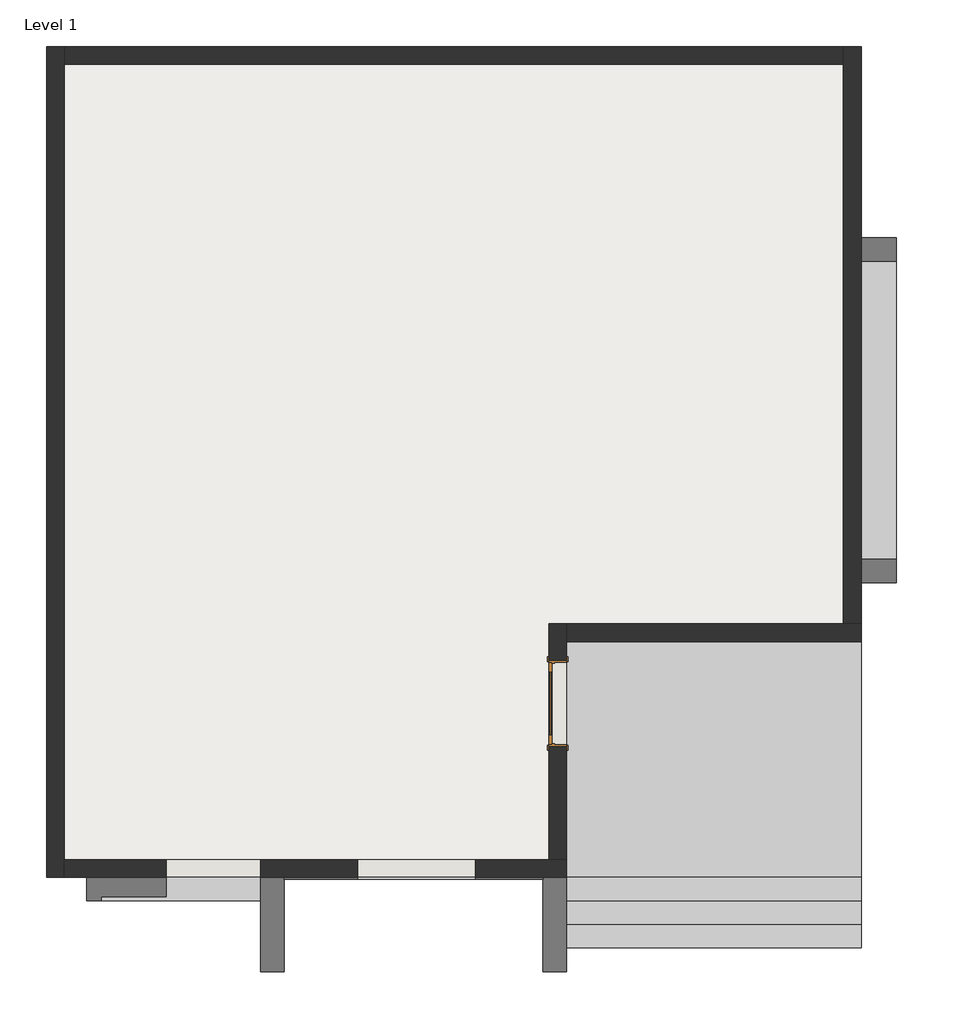
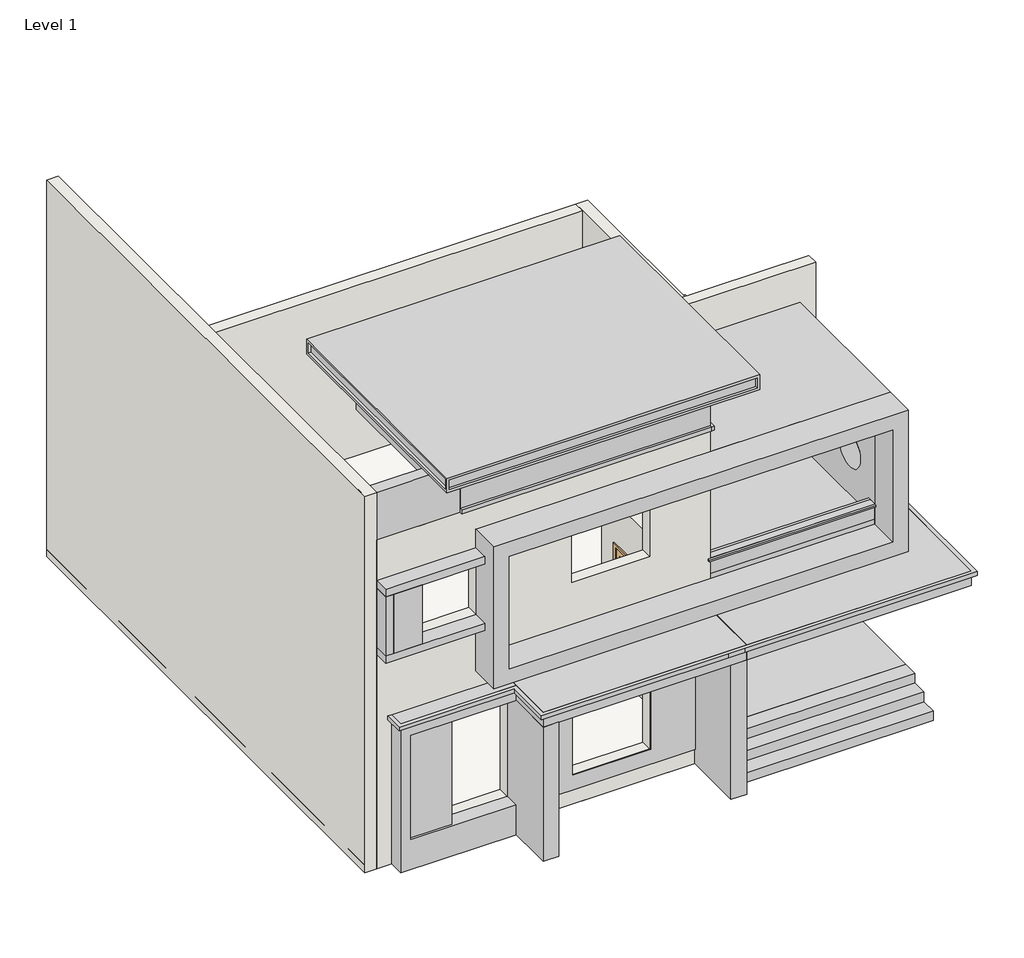
# One storey: 6 walls, 1 door, 1 proxy, 1 slab.
"""IFC4 building model written with IfcOpenShell, lengths in millimetres."""

from ifc_helpers import new_model, si_unit, origin, origin_with_axes, place, context, project, spatial, polyline, outline, extrude, faceted_brep, transform, mapped, element, save
from components import generic_models_1_generic_models_1_6c446dcb, door_103cf79b

model = new_model("IFC4")

# Units and contexts
model_context = context("Model", 3, world=origin())
ifc_project = project(units=[si_unit("LENGTHUNIT", "METRE", prefix="MILLI")], contexts=[model_context])

# Site, building, storey
site = spatial("IfcSite", under=ifc_project)
building = spatial("IfcBuilding", under=site)
storey = spatial("IfcBuildingStorey", under=building, Name="Level 1", Elevation=0.0)

# Proxy
placement = place(None, origin())
generic_models_1_generic_models_1_shape = generic_models_1_generic_models_1_6c446dcb(model_context)
element("IfcBuildingElementProxy", 1, Name="Generic Models 1 : Generic Models 1", ObjectType="Generic Models 1 : Generic Models 1", at=placement, inside=storey, context=model_context, shape_type="MappedRepresentation", body=[
    mapped(generic_models_1_generic_models_1_shape, transform((0.0, 0.0, 0.0), x_axis=(1.0, 0.0, 0.0), y_axis=(0.0, 1.0, 0.0), z_axis=(0.0, 0.0, 1.0))),
])

# Door
door_shape = door_103cf79b(model_context)
element("IfcDoor", 2, ObjectType="Door-Interior-Single-1_Panel-Wood : 3'6\" x 7'", at=placement, inside=storey, context=model_context, shape_type="MappedRepresentation", body=[
    mapped(door_shape, transform((-5484.7968714, -148.5569638, 609.6), x_axis=(0.0, 1.0, 0.0), y_axis=(-1.0, 0.0, 0.0), z_axis=(0.0, 0.0, 1.0))),
])

# Slab
element("IfcSlab", 3, ObjectType="6\" floor", at=placement, inside=storey, context=model_context, shape_type="SweptSolid", body=[
    extrude(outline(polyline([(-12098.3218714, 8347.7430362), (-1557.3218714, 8347.7430362), (-1557.3218714, 651.5430362), (-5367.3218714, 651.5430362), (-5367.3218714, -2396.4569638), (-12098.3218714, -2396.4569638), (-12098.3218714, 8347.7430362)])), origin_with_axes(), (0.0, 0.0, 1.0), 152.4),
])

# Walls
element("IfcWall", 4, ObjectType="9\" wall", at=placement, inside=storey, context=model_context, shape_type="Brep", body=[
    faceted_brep([(-12098.3218714, 8347.7430362, 7759.3157356), (-12098.3218714, 8347.7430362, 0.0), (-12098.3218714, -2396.4569638, 0.0), (-12098.3218714, -2396.4569638, 7759.3157356), (-11869.7218714, 8347.7430362, 0.0), (-11869.7218714, 8347.7430362, 3657.6), (-11869.7218714, 8347.7430362, 5621.6075521), (-11869.7218714, 8347.7430362, 7759.3157356), (-11869.7218714, -2396.4569638, 7759.3157356), (-11869.7218714, -2396.4569638, 6776.5796237), (-11869.7218714, -2396.4569638, 0.0), (-11869.7218714, -2167.8569638, 0.0), (-11869.7218714, 8119.1430362, 0.0)], [[[0, 1, 2, 3]], [[4, 5, 6, 7, 8, 9, 10, 11, 12]], [[2, 1, 4, 12, 11, 10]], [[0, 3, 8, 7]], [[3, 2, 10, 9, 8]], [[0, 7, 6, 5, 4, 1]]]),
])
element("IfcWall", 5, ObjectType="9\" wall", at=placement, inside=storey, context=model_context, shape_type="Brep", body=[
    faceted_brep([(-11869.7218714, -2396.4569638, 0.0), (-5367.3218714, -2396.4569638, 0.0), (-5367.3218714, -2396.4569638, 6776.5796237), (-11869.7218714, -2396.4569638, 6776.5796237), (-9329.7218714, -2396.4569638, 2743.2), (-9329.7218714, -2396.4569638, 609.6), (-10548.9218714, -2396.4569638, 609.6), (-10548.9218714, -2396.4569638, 2743.2), (-6548.4218714, -2396.4569638, 2743.2), (-6548.4218714, -2396.4569638, 609.6), (-8072.4218714, -2396.4569638, 609.6), (-8072.4218714, -2396.4569638, 2743.2), (-9939.3218714, -2396.4569638, 5791.2), (-9939.3218714, -2396.4569638, 4572.0), (-11158.5218714, -2396.4569638, 4572.0), (-11158.5218714, -2396.4569638, 5791.2), (-6548.4218714, -2396.4569638, 5791.2), (-6548.4218714, -2396.4569638, 4572.0), (-8072.4218714, -2396.4569638, 4572.0), (-8072.4218714, -2396.4569638, 5791.2), (-5367.3218714, -2167.8569638, 0.0), (-5595.9218714, -2167.8569638, 0.0), (-11869.7218714, -2167.8569638, 0.0), (-11869.7218714, -2167.8569638, 6776.5796237), (-5595.9218714, -2167.8569638, 6776.5796237), (-5367.3218714, -2167.8569638, 6776.5796237), (-9329.7218714, -2167.8569638, 609.6), (-9329.7218714, -2167.8569638, 2743.2), (-10548.9218714, -2167.8569638, 2743.2), (-10548.9218714, -2167.8569638, 609.6), (-6548.4218714, -2167.8569638, 609.6), (-6548.4218714, -2167.8569638, 2743.2), (-8072.4218714, -2167.8569638, 2743.2), (-8072.4218714, -2167.8569638, 609.6), (-9939.3218714, -2167.8569638, 4572.0), (-9939.3218714, -2167.8569638, 5791.2), (-11158.5218714, -2167.8569638, 5791.2), (-11158.5218714, -2167.8569638, 4572.0), (-6548.4218714, -2167.8569638, 4572.0), (-6548.4218714, -2167.8569638, 5791.2), (-8072.4218714, -2167.8569638, 5791.2), (-8072.4218714, -2167.8569638, 4572.0)], [[[0, 1, 2, 3], [4, 5, 6, 7], [8, 9, 10, 11], [12, 13, 14, 15], [16, 17, 18, 19]], [[20, 21, 22, 23, 24, 25], [26, 27, 28, 29], [30, 31, 32, 33], [34, 35, 36, 37], [38, 39, 40, 41]], [[1, 0, 22, 21, 20]], [[3, 2, 25, 24, 23]], [[0, 3, 23, 22]], [[2, 1, 20, 25]], [[26, 5, 4, 27]], [[28, 7, 6, 29]], [[5, 26, 29, 6]], [[30, 9, 8, 31]], [[10, 33, 32, 11]], [[9, 30, 33, 10]], [[31, 8, 11, 32]], [[7, 28, 27, 4]], [[34, 13, 12, 35]], [[35, 12, 15, 36]], [[36, 15, 14, 37]], [[13, 34, 37, 14]], [[38, 17, 16, 39]], [[18, 41, 40, 19]], [[17, 38, 41, 18]], [[19, 40, 39, 16]]]),
])
element("IfcWall", 6, ObjectType="9\" wall", at=placement, inside=storey, context=model_context, shape_type="Brep", body=[
    faceted_brep([(-5367.3218714, -2167.8569638, 0.0), (-5367.3218714, 651.5430362, 0.0), (-5367.3218714, 880.1430362, 0.0), (-5367.3218714, 880.1430362, 6776.5796237), (-5367.3218714, -2167.8569638, 6776.5796237), (-5367.3218714, 410.2430362, 2768.6), (-5367.3218714, 410.2430362, 609.6), (-5367.3218714, -707.3569638, 609.6), (-5367.3218714, -707.3569638, 2768.6), (-5367.3218714, 410.2430362, 5816.6), (-5367.3218714, 410.2430362, 3657.6), (-5367.3218714, -707.3569638, 3657.6), (-5367.3218714, -707.3569638, 5816.6), (-5595.9218714, 880.1430362, 0.0), (-5595.9218714, -2167.8569638, 0.0), (-5595.9218714, -2167.8569638, 6776.5796237), (-5595.9218714, 880.1430362, 6776.5796237), (-5595.9218714, 410.2430362, 609.6), (-5595.9218714, 410.2430362, 2768.6), (-5595.9218714, -707.3569638, 2768.6), (-5595.9218714, -707.3569638, 609.6), (-5595.9218714, 410.2430362, 3657.6), (-5595.9218714, 410.2430362, 5816.6), (-5595.9218714, -707.3569638, 5816.6), (-5595.9218714, -707.3569638, 3657.6)], [[[0, 1, 2, 3, 4], [5, 6, 7, 8], [9, 10, 11, 12]], [[13, 14, 15, 16], [17, 18, 19, 20], [21, 22, 23, 24]], [[2, 1, 0, 14, 13]], [[4, 3, 16, 15]], [[0, 4, 15, 14]], [[3, 2, 13, 16]], [[17, 6, 5, 18]], [[18, 5, 8, 19]], [[19, 8, 7, 20]], [[6, 17, 20, 7]], [[22, 21, 10, 9]], [[23, 22, 9, 12]], [[24, 23, 12, 11]], [[21, 24, 11, 10]]]),
])
element("IfcWall", 7, ObjectType="9\" wall", at=placement, inside=storey, context=model_context, shape_type="Brep", body=[
    faceted_brep([(-5367.3218714, 651.5430362, 0.0), (-1557.3218714, 651.5430362, 0.0), (-1557.3218714, 651.5430362, 7046.341498), (-5367.3218714, 651.5430362, 7046.341498), (-5367.3218714, 880.1430362, 0.0), (-5367.3218714, 880.1430362, 6776.5796237), (-5367.3218714, 880.1430362, 7046.341498), (-1557.3218714, 880.1430362, 7046.341498), (-1557.3218714, 880.1430362, 5621.6075521), (-1557.3218714, 880.1430362, 3657.6), (-1557.3218714, 880.1430362, 0.0), (-1785.9218714, 880.1430362, 0.0)], [[[0, 1, 2, 3]], [[4, 5, 6, 7, 8, 9, 10, 11]], [[1, 0, 4, 11, 10]], [[3, 2, 7, 6]], [[0, 3, 6, 5, 4]], [[1, 10, 9, 8, 7, 2]]]),
])
element("IfcWall", 8, ObjectType="9\" wall", at=placement, inside=storey, context=model_context, shape_type="Brep", body=[
    faceted_brep([(-1557.3218714, 880.1430362, 0.0), (-1557.3218714, 8347.7430362, 0.0), (-1557.3218714, 8347.7430362, 3657.6), (-1557.3218714, 8119.1430362, 3657.6), (-1557.3218714, 880.1430362, 3657.6), (-1785.9218714, 880.1430362, 0.0), (-1785.9218714, 880.1430362, 3657.6), (-1785.9218714, 8119.1430362, 3657.6), (-1785.9218714, 8347.7430362, 3657.6), (-1785.9218714, 8347.7430362, 0.0), (-1785.9218714, 8119.1430362, 0.0)], [[[0, 1, 2, 3, 4]], [[5, 6, 7, 8, 9, 10]], [[1, 0, 5, 10, 9]], [[4, 3, 2, 8, 7, 6]], [[0, 4, 6, 5]], [[2, 1, 9, 8]]]),
])
element("IfcWall", 9, ObjectType="9\" wall", at=placement, inside=storey, context=model_context, shape_type="SweptSolid", body=[
    extrude(outline(polyline([(-11869.7218714, 8347.7430362), (-1785.9218714, 8347.7430362), (-1785.9218714, 8119.1430362), (-11869.7218714, 8119.1430362), (-11869.7218714, 8347.7430362)])), origin_with_axes(), (0.0, 0.0, 1.0), 3657.6),
])

save(model, "model.ifc")

# Revit data of these elements
# Type "Door-Interior-Single-1_Panel-Wood : 3'6\" x 7'"
#   Type Mark = "9"
#   Assembly Code = "C1020300"
#   Analytic Construction = "Wooden"
#   Top Rail = 0' - 4 11/16"
#   Thickness = 0' - 1 3/8"
#   Thermal Resistance (R) = 2.5876 (h·ft²·°F)/BTU
#   Swing Angle [instance default] = 90.00°
#   Stiles = 0' - 4 3/4"
#   Rough Width = 3' - 8"
#   Rough Height = 7' - 1"
#   Height = 7' - 0"
#   Width = 3' - 6"
#   Heat Transfer Coefficient (U) = 0.3865 BTU/(h·ft²·°F)
#   Bottom Rail = 0' - 9 1/8"
#   Trim Material = Cherry
#   Panel Material = Cherry
#   Frame Material = Cherry
#   Door Handle Material = Aluminum
#   Visual Light Transmittance = 0
#   Solar Heat Gain Coefficient = 0
#   Wall Closure = (empty or 0)
#   Function = (empty or 0)
# Type "6\" floor"
#   Assembly Code = "B1010"
#   Function = 0
#   Layers, outside or top first: 0' - 6" no material (function 1)
# Type "9\" wall"
#   Assembly Code = "B2010"
#   Layers, outside or top first: 0' - 9" "ash" (function 1)
# Element 1 (IfcBuildingElementProxy, "Generic Models 1 : Generic Models 1")
#   Phase Created = New Construction
#   Materials on its faces: "Gypsum Wall Board", "Earth", "Wood - Stained", "wood colour", "wall wood"
# Element 2 (IfcDoor, "Door-Interior-Single-1_Panel-Wood : 3'6\" x 7'")
#   Swing Angle = 90.00°
#   Phase Created = New Construction
#   Materials on its faces: "Cherry", "Aluminum"
# Element 3 (IfcSlab, "6\" floor")
#   built-in parameter 1001955 = 3.14159 (stored number, unit not read)
#   Height Offset From Level = 0' - 6"
#   Phase Created = New Construction
#   Materials on its faces: "Default Floor"
# Element 4 (IfcWall, "9\" wall")
#   Top Offset = 13' - 5.48487"
#   Base Offset = 0' - 0"
#   wall height = 25' - 5.48487"
#   Phase Created = New Construction
#   Base Constraint = Level 1
#   Top Constraint = Level 3
#   Materials on its faces: "ash"
# Elements 5, 6 (IfcWall, "9\" wall")
#   Top Offset = 10' - 2.79447"
#   Base Offset = 0' - 0"
#   wall height = 22' - 2.79447"
#   Phase Created = New Construction
#   Base Constraint = Level 1
#   Top Constraint = Level 3
#   Materials on its faces: "ash"
# Element 7 (IfcWall, "9\" wall")
#   Top Offset = 11' - 1.41502"
#   Base Offset = 0' - 0"
#   wall height = 23' - 1.41502"
#   Phase Created = New Construction
#   Base Constraint = Level 1
#   Top Constraint = Level 3
#   Materials on its faces: "ash"
# Elements 8, 9 (IfcWall, "9\" wall")
#   Top Offset = 0' - 0"
#   Base Offset = 0' - 0"
#   wall height = 12' - 0"
#   Phase Created = New Construction
#   Base Constraint = Level 1
#   Top Constraint = Level 3
#   Materials on its faces: "ash"
# Materials
#   "Cherry": class "Wood", colour RGB 226 177 128, transparency 0, Description = "Prunus Serotina", Cost = 0
#   "Aluminum": class "Metal", colour RGB 247 247 247, transparency 0, Description = "Aluminum 6061", Cost = 0
#   "ash": class "Generic", colour RGB 120 120 120, transparency 0, Cost = 0
#   "Gypsum Wall Board": class "Generic", colour RGB 127 127 127, transparency 0, Description = "Gypsum Wall Board", Cost = 0
#   "Earth": class "Generic", colour RGB 97 75 62, transparency 0, Description = "Soil", Cost = 0
#   "Wood - Stained": class "Wood", colour RGB 224 178 126, transparency 0, Cost = 0
#   "wood colour": class "Generic", colour RGB 120 120 120, transparency 0, Cost = 0
#   "wall wood": class "Generic", colour RGB 120 120 120, transparency 0, Cost = 0
#   "Default Floor": colour RGB 128 128 128, transparency 0, Cost = 0
